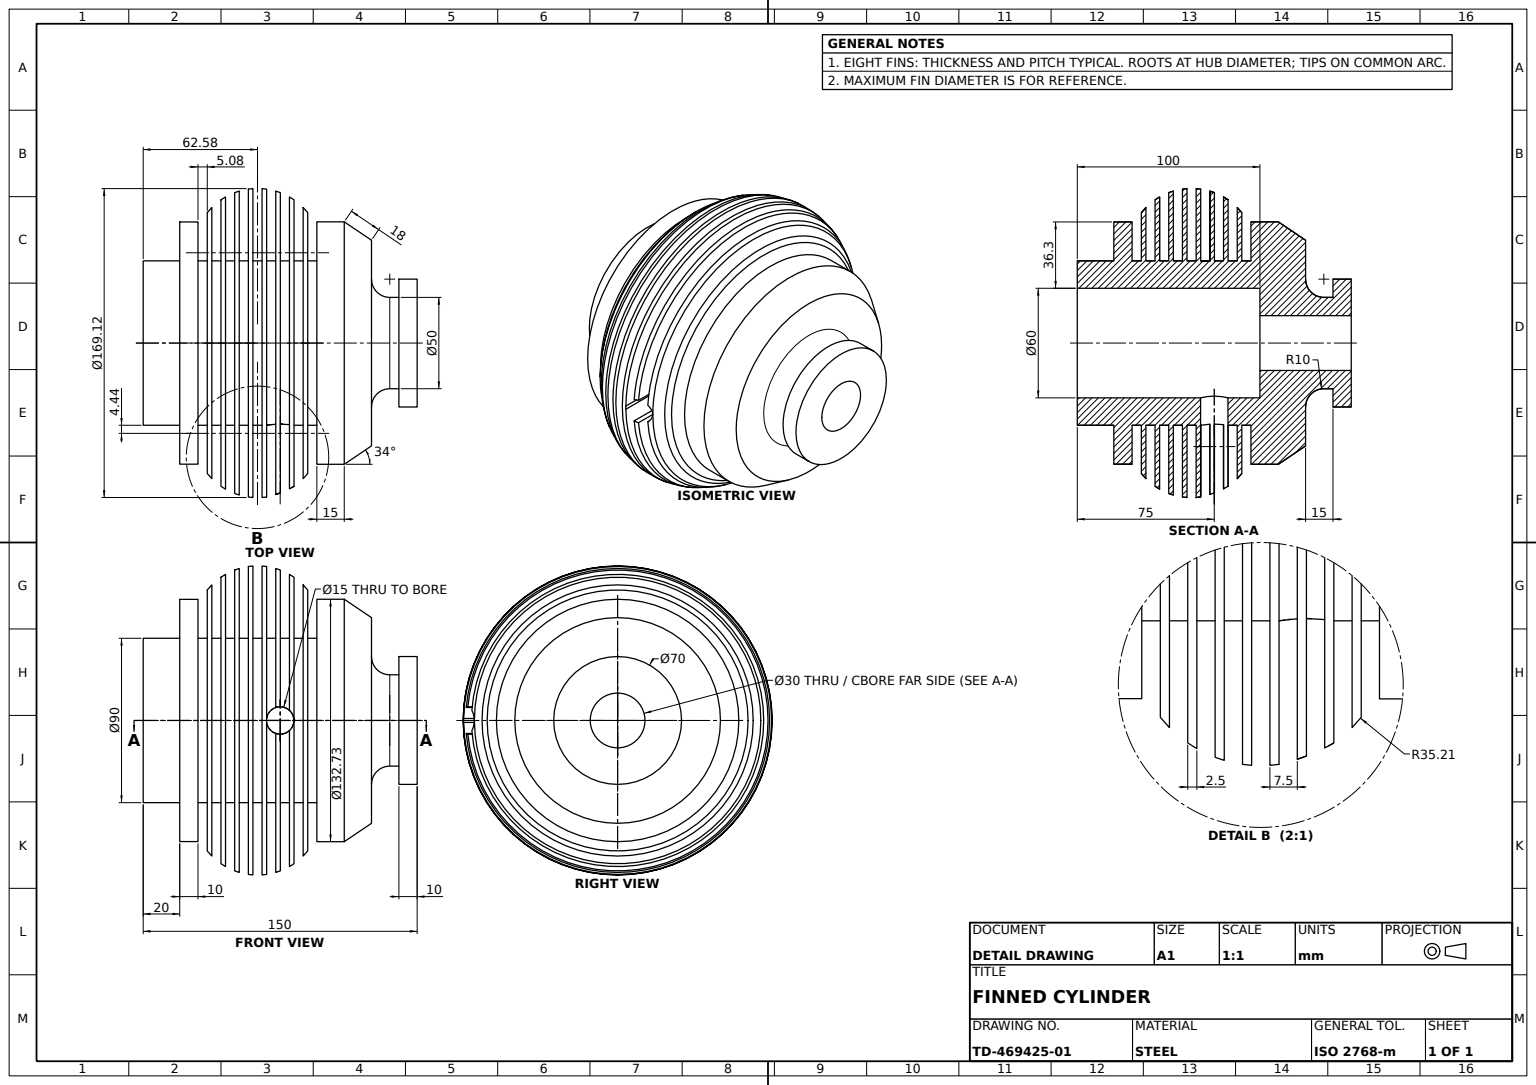
SolidWorks part; units mm, degrees
material "Plain Carbon Steel"
ref_plane "Front Plane" through (0, 0, 0) normal (0, 0, 1) x (1, 0, 0)
ref_plane "Top Plane" through (0, 0, 0) normal (0, 1, 0) x (1, 0, 0)
ref_plane "Right Plane" through (0, 0, 0) normal (1, 0, 0) x (0, 0, -1)
sketch "Finned Body Profile" plane through (0, 0, 0) normal (0, 0, 1) x (1, 0, 0)
  line L0 (-190.2903, -11.8639) -> (185.6042, -11.8639) construction
  line L1 (-2.3431, 3.1361) -> (-2.3431, 23.1361)
  line L2 (-2.3431, 23.1361) -> (7.6569, 23.1361)
  line L3 (7.6569, 23.1361) -> (7.6569, 13.1361)
  line L4 (22.6569, 23.1361) -> (22.6569, 44.4361)
  line L5 (22.6569, 44.4361) -> (37.5796, 54.5016)
  line L6 (37.5796, 54.5016) -> (52.5796, 54.5016)
  line L7 (52.5796, 54.5016) -> (52.5796, 33.1361)
  line L8 (52.5796, 33.1361) -> (57.5796, 33.1361)
  line L9 (-2.3431, 3.1361) -> (47.6569, 3.1361)
  line L10 (52.5796, 33.1361) -> (117.6569, 33.1361) construction
  line L11 (47.6569, 3.1361) -> (47.6569, 18.1361)
  line L12 (47.6569, 18.1361) -> (147.6569, 18.1361)
  line L13 (147.6569, 18.1361) -> (147.6569, 33.1361)
  line L14 (147.6569, 33.1361) -> (127.6569, 33.1361)
  line L15 (127.6569, 33.1361) -> (127.6569, 54.4361)
  line L16 (127.6569, 54.4361) -> (117.6569, 54.4361)
  line L17 (117.6569, 54.4361) -> (117.6569, 33.1361)
  line L18 (7.6569, 13.1361) -> (12.6569, 13.1361)
  line L19 (57.5796, 33.1361) -> (57.5796, 59.5597)
  line L20 (60.0796, 62.3658) -> (60.0796, 33.1361)
  line L21 (65.0796, 33.1361) -> (65.0796, 66.5507)
  line L22 (67.5796, 68.1257) -> (67.5796, 33.1361)
  line L23 (72.5796, 70.4893) -> (72.5796, 33.1361)
  line L24 (75.0796, 71.333) -> (75.0796, 33.1361)
  line L25 (80.0796, 72.4262) -> (80.0796, 33.1361)
  line L26 (82.5796, 72.6941) -> (82.5796, 33.1361)
  line L35 (60.0796, 33.1361) -> (65.0796, 33.1361)
  line L36 (67.5796, 33.1361) -> (72.5796, 33.1361)
  line L37 (75.0796, 33.1361) -> (80.0796, 33.1361)
  line L38 (82.5796, 33.1361) -> (87.5796, 33.1361)
  line L43 (85.0796, 37.5761) -> (85.0796, 82.9644) construction
  line L44 (112.5796, 33.1361) -> (117.6569, 33.1361)
  line L45 (95.0796, 33.1361) -> (90.0796, 33.1361)
  line L46 (102.5796, 33.1361) -> (97.5796, 33.1361)
  line L47 (110.0796, 33.1361) -> (105.0796, 33.1361)
  line L48 (87.5796, 72.6941) -> (87.5796, 33.1361)
  line L49 (90.0796, 72.4262) -> (90.0796, 33.1361)
  line L50 (95.0796, 71.333) -> (95.0796, 33.1361)
  line L51 (97.5796, 70.4893) -> (97.5796, 33.1361)
  line L52 (102.5796, 68.1257) -> (102.5796, 33.1361)
  line L53 (105.0796, 33.1361) -> (105.0796, 66.5507)
  line L54 (110.0796, 62.3658) -> (110.0796, 33.1361)
  line L55 (112.5796, 33.1361) -> (112.5796, 59.5597)
  arc A0 (22.6569, 23.1361) -> (12.6569, 13.1361) centre (12.6569, 23.1361) cw
  arc A1 (57.5796, 59.5597) -> (60.0796, 62.3658) centre (85.0796, 37.5761) cw
  arc A2 (65.0796, 66.5507) -> (67.5796, 68.1257) centre (85.0796, 37.5761) cw
  arc A3 (72.5796, 70.4893) -> (75.0796, 71.333) centre (85.0796, 37.5761) cw
  arc A4 (80.0796, 72.4262) -> (82.5796, 72.6941) centre (85.0796, 37.5761) cw
  arc A9 (90.0796, 72.4262) -> (87.5796, 72.6941) centre (85.0796, 37.5761) ccw
  arc A10 (97.5796, 70.4893) -> (95.0796, 71.333) centre (85.0796, 37.5761) ccw
  arc A11 (105.0796, 66.5507) -> (102.5796, 68.1257) centre (85.0796, 37.5761) ccw
  arc A12 (112.5796, 59.5597) -> (110.0796, 62.3658) centre (85.0796, 37.5761) ccw
  point P4 (-2.3431, -11.8639)
  point P18 (-2.3431, -11.8639)
  point P29 (22.6569, 13.1361)
  dimension "D1" = 100
  dimension "D13" = 21.3
  dimension "D16" = 10
  dimension "D19" = 2.5
  dimension "D30" = 35.207
  dimension "D2" = 50
  dimension "D3" = 15
  dimension "D4" = 20
  dimension "D5" = 10
  dimension "D6" = 5
  dimension "D7" = 146
  dimension "D8" = 18
  dimension "D9" = 15
  dimension "D10" = 10
  dimension "D11" = 20
  dimension "D12" = 10
  dimension "D14" = 36.3
  dimension "D15" = 15
  dimension "D17" = 5
  dimension "D18" = 15
  dimension "D20" = 2.5
  dimension "D21" = 2.5
  dimension "D22" = 5
  dimension "D23" = 5
  dimension "D24" = 5
  dimension "D25" = 5
  dimension "D26" = 2.3431
  dimension "D27" = 11.8639
  dimension "D28" = 2.5
  dimension "D29" = 375.8945
  dimension "D31" = 4.44
revolve "Finned Body Revolve" add sketch "Finned Body Profile" angle 360 about L0
sketch "Through Bore Profile" plane through (0, 0, 0) normal (0, 0, 1) x (1, 0, 0)
  line L0 (47.6569, -11.8639) -> (-2.3431, -11.8639) construction
  line L9 (147.6569, -56.8639) -> (147.6569, 33.1361) construction
  circle A0 centre (72.6569, -11.8639) radius 7.5
  dimension "D1" = 15
  dimension "D2" = 0
  dimension "D3" = 75
extrude "Through Bore" cut sketch "Through Bore Profile" against normal blind 113
